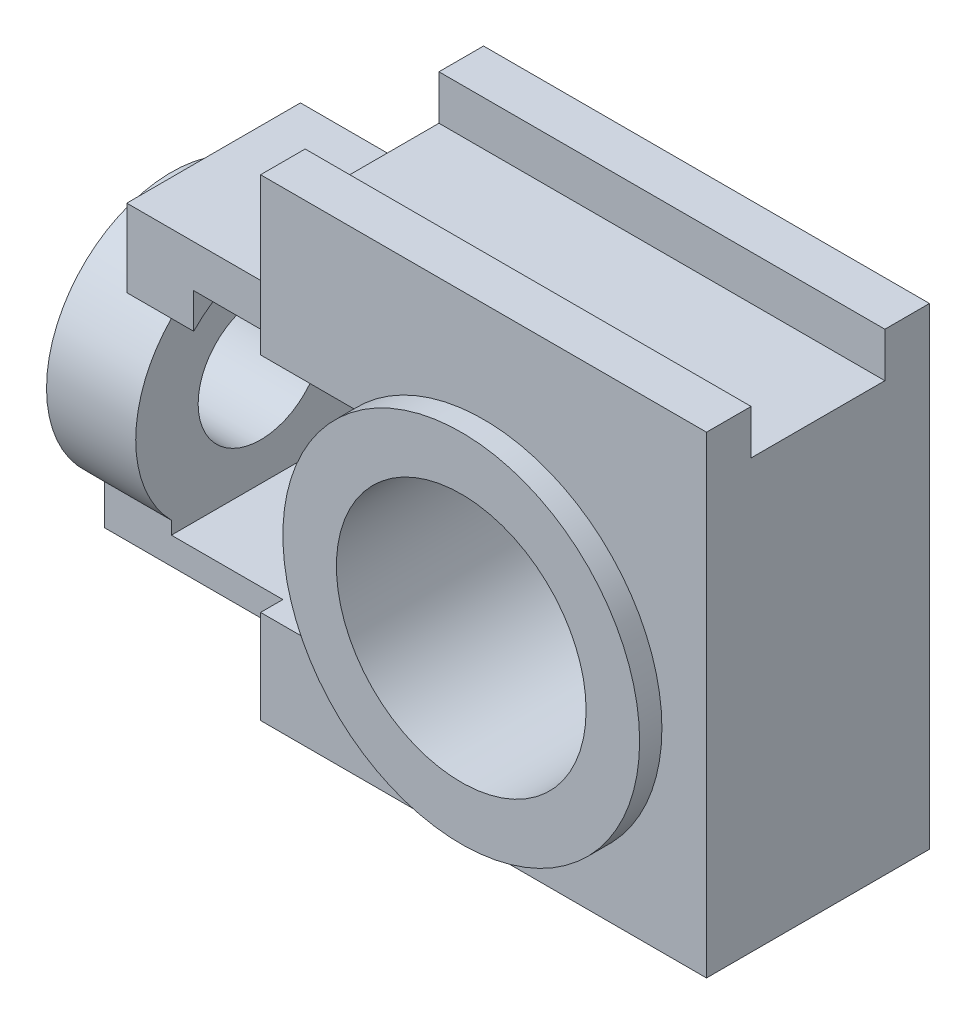
ISO-10303-21;
HEADER;
FILE_DESCRIPTION(('STEP AP214'),'2;1');
FILE_NAME('part.step','',(''),(''),'','','');
FILE_SCHEMA(('AUTOMOTIVE_DESIGN { 1 0 10303 214 1 1 1 1 }'));
ENDSEC;
DATA;
#1=APPLICATION_CONTEXT('core data for automotive mechanical design processes');
#2=APPLICATION_PROTOCOL_DEFINITION('international standard','automotive_design',2000,#1);
#3=PRODUCT_CONTEXT('',#1,'mechanical');
#4=PRODUCT('Part','Part','',(#3));
#5=PRODUCT_RELATED_PRODUCT_CATEGORY('part','',(#4));
#6=PRODUCT_DEFINITION_FORMATION('','',#4);
#7=PRODUCT_DEFINITION_CONTEXT('part definition',#1,'design');
#8=PRODUCT_DEFINITION('design','',#6,#7);
#9=PRODUCT_DEFINITION_SHAPE('','',#8);
#10=(LENGTH_UNIT() NAMED_UNIT(*) SI_UNIT(.MILLI.,.METRE.));
#11=(NAMED_UNIT(*) PLANE_ANGLE_UNIT() SI_UNIT($,.RADIAN.));
#12=(NAMED_UNIT(*) SI_UNIT($,.STERADIAN.) SOLID_ANGLE_UNIT());
#13=UNCERTAINTY_MEASURE_WITH_UNIT(LENGTH_MEASURE(1.E-05),#10,'distance_accuracy_value','');
#14=(GEOMETRIC_REPRESENTATION_CONTEXT(3) GLOBAL_UNCERTAINTY_ASSIGNED_CONTEXT((#13)) GLOBAL_UNIT_ASSIGNED_CONTEXT((#10,
#11,#12)) REPRESENTATION_CONTEXT('',''));
#15=CARTESIAN_POINT('',(0.,0.,0.));
#16=DIRECTION('',(0.,0.,1.));
#17=DIRECTION('',(1.,0.,0.));
#18=AXIS2_PLACEMENT_3D('',#15,#16,#17);
#19=CARTESIAN_POINT('',(0.,21.,0.));
#20=DIRECTION('',(0.,1.,0.));
#21=DIRECTION('',(0.,0.,1.));
#22=AXIS2_PLACEMENT_3D('',#19,#20,#21);
#23=PLANE('',#22);
#24=DIRECTION('',(1.,0.,0.));
#25=VECTOR('',#24,1.);
#26=CARTESIAN_POINT('',(-90.,21.,-20.));
#27=LINE('',#26,#25);
#28=CARTESIAN_POINT('',(-75.,21.,-20.));
#29=VERTEX_POINT('',#28);
#30=CARTESIAN_POINT('',(-50.,21.,-20.));
#31=VERTEX_POINT('',#30);
#32=EDGE_CURVE('E417',#29,#31,#27,.T.);
#33=ORIENTED_EDGE('',*,*,#32,.F.);
#34=DIRECTION('',(0.,0.,1.));
#35=VECTOR('',#34,1.);
#36=CARTESIAN_POINT('',(-75.,21.,0.));
#37=LINE('',#36,#35);
#38=CARTESIAN_POINT('',(-75.,21.,20.));
#39=VERTEX_POINT('',#38);
#40=EDGE_CURVE('E446',#29,#39,#37,.T.);
#41=ORIENTED_EDGE('',*,*,#40,.T.);
#42=DIRECTION('',(1.,0.,0.));
#43=VECTOR('',#42,1.);
#44=CARTESIAN_POINT('',(-90.,21.,20.));
#45=LINE('',#44,#43);
#46=CARTESIAN_POINT('',(-50.,21.,20.));
#47=VERTEX_POINT('',#46);
#48=EDGE_CURVE('E252',#39,#47,#45,.T.);
#49=ORIENTED_EDGE('',*,*,#48,.T.);
#50=DIRECTION('',(0.,0.,1.));
#51=VECTOR('',#50,1.);
#52=CARTESIAN_POINT('',(-50.,21.,-25.));
#53=LINE('',#52,#51);
#54=CARTESIAN_POINT('',(-50.,21.,25.));
#55=VERTEX_POINT('',#54);
#56=EDGE_CURVE('E423',#47,#55,#53,.T.);
#57=ORIENTED_EDGE('',*,*,#56,.T.);
#58=DIRECTION('',(1.,0.,0.));
#59=VECTOR('',#58,1.);
#60=CARTESIAN_POINT('',(-50.,21.,25.));
#61=LINE('',#60,#59);
#62=CARTESIAN_POINT('',(-33.0718913883074,21.,25.));
#63=VERTEX_POINT('',#62);
#64=EDGE_CURVE('E428',#55,#63,#61,.T.);
#65=ORIENTED_EDGE('',*,*,#64,.T.);
#66=DIRECTION('',(0.,0.,1.));
#67=VECTOR('',#66,1.);
#68=CARTESIAN_POINT('',(-33.0718913883074,21.,-25.));
#69=LINE('',#68,#67);
#70=CARTESIAN_POINT('',(-33.0718913883074,21.,-25.));
#71=VERTEX_POINT('',#70);
#72=EDGE_CURVE('E452',#71,#63,#69,.T.);
#73=ORIENTED_EDGE('',*,*,#72,.F.);
#74=DIRECTION('',(-1.,0.,0.));
#75=VECTOR('',#74,1.);
#76=CARTESIAN_POINT('',(50.,21.,-25.));
#77=LINE('',#76,#75);
#78=CARTESIAN_POINT('',(-50.,21.,-25.));
#79=VERTEX_POINT('',#78);
#80=EDGE_CURVE('E416',#71,#79,#77,.T.);
#81=ORIENTED_EDGE('',*,*,#80,.T.);
#82=EDGE_CURVE('E421',#79,#31,#53,.T.);
#83=ORIENTED_EDGE('',*,*,#82,.T.);
#84=EDGE_LOOP('',(#33,#41,#49,#57,#65,#73,#81,#83));
#85=FACE_BOUND('',#84,.T.);
#86=ADVANCED_FACE('F50',(#85),#23,.T.);
#87=CARTESIAN_POINT('',(-50.,106.,-25.));
#88=DIRECTION('',(-1.,0.,0.));
#89=DIRECTION('',(0.,-1.,0.));
#90=AXIS2_PLACEMENT_3D('',#87,#88,#89);
#91=PLANE('',#90);
#92=DIRECTION('',(0.,0.,1.));
#93=VECTOR('',#92,1.);
#94=CARTESIAN_POINT('',(-50.,71.,-25.));
#95=LINE('',#94,#93);
#96=CARTESIAN_POINT('',(-50.,71.,-19.0946483751058));
#97=VERTEX_POINT('',#96);
#98=CARTESIAN_POINT('',(-50.,71.,20.));
#99=VERTEX_POINT('',#98);
#100=EDGE_CURVE('E368',#97,#99,#95,.T.);
#101=ORIENTED_EDGE('',*,*,#100,.T.);
#102=DIRECTION('',(0.,-0.00096236717076537,0.999999536924607));
#103=VECTOR('',#102,1.);
#104=CARTESIAN_POINT('',(-50.,71.,20.));
#105=LINE('',#104,#103);
#106=CARTESIAN_POINT('',(-50.,71.0142498881101,5.19288485281843));
#107=VERTEX_POINT('',#106);
#108=EDGE_CURVE('E262',#107,#99,#105,.T.);
#109=ORIENTED_EDGE('',*,*,#108,.F.);
#110=CARTESIAN_POINT('',(-50.,43.5,0.));
#111=DIRECTION('',(1.,0.,0.));
#112=DIRECTION('',(0.,-1.,0.));
#113=AXIS2_PLACEMENT_3D('',#110,#111,#112);
#114=CIRCLE('',#113,28.);
#115=CARTESIAN_POINT('',(-50.,71.0142498881101,-5.19288485281842));
#116=VERTEX_POINT('',#115);
#117=EDGE_CURVE('E304',#116,#107,#114,.T.);
#118=ORIENTED_EDGE('',*,*,#117,.F.);
#119=DIRECTION('',(0.,0.00102504121876831,0.999999474645112));
#120=VECTOR('',#119,1.);
#121=CARTESIAN_POINT('',(-50.,71.,-19.0946483751058));
#122=LINE('',#121,#120);
#123=EDGE_CURVE('E266',#97,#116,#122,.T.);
#124=ORIENTED_EDGE('',*,*,#123,.F.);
#125=EDGE_LOOP('',(#101,#109,#118,#124));
#126=FACE_BOUND('',#125,.T.);
#127=ADVANCED_FACE('F506',(#126),#91,.T.);
#128=CARTESIAN_POINT('',(-50.,71.,-25.));
#129=VERTEX_POINT('',#128);
#130=EDGE_CURVE('E362',#129,#97,#95,.T.);
#131=ORIENTED_EDGE('',*,*,#130,.T.);
#132=DIRECTION('',(0.,-0.999869604471374,-0.0161485000621516));
#133=VECTOR('',#132,1.);
#134=CARTESIAN_POINT('',(-50.,80.4842706996611,-18.9414716555636));
#135=LINE('',#134,#133);
#136=CARTESIAN_POINT('',(-50.,80.4842706996611,-18.9414716555636));
#137=VERTEX_POINT('',#136);
#138=EDGE_CURVE('E305',#137,#97,#135,.T.);
#139=ORIENTED_EDGE('',*,*,#138,.F.);
#140=DIRECTION('',(0.,0.,-1.));
#141=VECTOR('',#140,1.);
#142=CARTESIAN_POINT('',(-50.,80.4842706996611,20.));
#143=LINE('',#142,#141);
#144=CARTESIAN_POINT('',(-50.,80.4842706996611,20.));
#145=VERTEX_POINT('',#144);
#146=EDGE_CURVE('E275',#145,#137,#143,.T.);
#147=ORIENTED_EDGE('',*,*,#146,.F.);
#148=DIRECTION('',(0.,1.,0.));
#149=VECTOR('',#148,1.);
#150=CARTESIAN_POINT('',(-50.,63.0959179422654,20.));
#151=LINE('',#150,#149);
#152=EDGE_CURVE('E293',#99,#145,#151,.T.);
#153=ORIENTED_EDGE('',*,*,#152,.F.);
#154=CARTESIAN_POINT('',(-50.,71.,25.));
#155=VERTEX_POINT('',#154);
#156=EDGE_CURVE('E367',#99,#155,#95,.T.);
#157=ORIENTED_EDGE('',*,*,#156,.T.);
#158=DIRECTION('',(0.,-1.,0.));
#159=VECTOR('',#158,1.);
#160=CARTESIAN_POINT('',(-50.,106.,25.));
#161=LINE('',#160,#159);
#162=CARTESIAN_POINT('',(-50.,106.,25.));
#163=VERTEX_POINT('',#162);
#164=EDGE_CURVE('E358',#163,#155,#161,.T.);
#165=ORIENTED_EDGE('',*,*,#164,.F.);
#166=DIRECTION('',(0.,0.,1.));
#167=VECTOR('',#166,1.);
#168=CARTESIAN_POINT('',(-50.,106.,-25.));
#169=LINE('',#168,#167);
#170=CARTESIAN_POINT('',(-50.,106.,15.));
#171=VERTEX_POINT('',#170);
#172=EDGE_CURVE('E373',#171,#163,#169,.T.);
#173=ORIENTED_EDGE('',*,*,#172,.F.);
#174=DIRECTION('',(0.,-1.,0.));
#175=VECTOR('',#174,1.);
#176=CARTESIAN_POINT('',(-50.,106.,15.));
#177=LINE('',#176,#175);
#178=CARTESIAN_POINT('',(-50.,96.,15.));
#179=VERTEX_POINT('',#178);
#180=EDGE_CURVE('E454',#171,#179,#177,.T.);
#181=ORIENTED_EDGE('',*,*,#180,.T.);
#182=DIRECTION('',(0.,0.,-1.));
#183=VECTOR('',#182,1.);
#184=CARTESIAN_POINT('',(-50.,96.,-25.));
#185=LINE('',#184,#183);
#186=CARTESIAN_POINT('',(-50.,96.,-15.));
#187=VERTEX_POINT('',#186);
#188=EDGE_CURVE('E54',#179,#187,#185,.T.);
#189=ORIENTED_EDGE('',*,*,#188,.T.);
#190=DIRECTION('',(0.,1.,0.));
#191=VECTOR('',#190,1.);
#192=CARTESIAN_POINT('',(-50.,106.,-15.));
#193=LINE('',#192,#191);
#194=CARTESIAN_POINT('',(-50.,106.,-15.));
#195=VERTEX_POINT('',#194);
#196=EDGE_CURVE('E11',#187,#195,#193,.T.);
#197=ORIENTED_EDGE('',*,*,#196,.T.);
#198=CARTESIAN_POINT('',(-50.,106.,-25.));
#199=VERTEX_POINT('',#198);
#200=EDGE_CURVE('E369',#199,#195,#169,.T.);
#201=ORIENTED_EDGE('',*,*,#200,.F.);
#202=DIRECTION('',(0.,-1.,0.));
#203=VECTOR('',#202,1.);
#204=CARTESIAN_POINT('',(-50.,106.,-25.));
#205=LINE('',#204,#203);
#206=EDGE_CURVE('E347',#199,#129,#205,.T.);
#207=ORIENTED_EDGE('',*,*,#206,.T.);
#208=EDGE_LOOP('',(#131,#139,#147,#153,#157,#165,#173,#181,#189,#197,#201,#207));
#209=FACE_BOUND('',#208,.T.);
#210=ADVANCED_FACE('F460',(#209),#91,.T.);
#211=CARTESIAN_POINT('',(-75.,43.5,0.));
#212=DIRECTION('',(-1.,0.,0.));
#213=DIRECTION('',(0.,0.,1.));
#214=AXIS2_PLACEMENT_3D('',#211,#212,#213);
#215=CYLINDRICAL_SURFACE('',#214,28.);
#216=DIRECTION('',(-1.,0.,0.));
#217=VECTOR('',#216,1.);
#218=CARTESIAN_POINT('',(-75.,23.9040820577346,20.));
#219=LINE('',#218,#217);
#220=CARTESIAN_POINT('',(-75.,23.9040820577346,20.));
#221=VERTEX_POINT('',#220);
#222=CARTESIAN_POINT('',(-90.,23.9040820577346,20.));
#223=VERTEX_POINT('',#222);
#224=EDGE_CURVE('E239',#221,#223,#219,.T.);
#225=ORIENTED_EDGE('',*,*,#224,.F.);
#226=CARTESIAN_POINT('',(-75.,43.5,0.));
#227=DIRECTION('',(-1.,0.,0.));
#228=DIRECTION('',(0.,0.,1.));
#229=AXIS2_PLACEMENT_3D('',#226,#227,#228);
#230=CIRCLE('',#229,28.);
#231=CARTESIAN_POINT('',(-75.,63.0959179422654,20.));
#232=VERTEX_POINT('',#231);
#233=EDGE_CURVE('E226',#221,#232,#230,.T.);
#234=ORIENTED_EDGE('',*,*,#233,.T.);
#235=DIRECTION('',(1.,0.,0.));
#236=VECTOR('',#235,1.);
#237=CARTESIAN_POINT('',(-85.,63.0959179422654,20.));
#238=LINE('',#237,#236);
#239=CARTESIAN_POINT('',(-85.,63.0959179422654,20.));
#240=VERTEX_POINT('',#239);
#241=EDGE_CURVE('E312',#240,#232,#238,.T.);
#242=ORIENTED_EDGE('',*,*,#241,.F.);
#243=CARTESIAN_POINT('',(-85.,43.5,0.));
#244=DIRECTION('',(1.,0.,0.));
#245=DIRECTION('',(0.,-1.,0.));
#246=AXIS2_PLACEMENT_3D('',#243,#244,#245);
#247=CIRCLE('',#246,28.);
#248=CARTESIAN_POINT('',(-85.,63.8711614859976,-19.2097834373896));
#249=VERTEX_POINT('',#248);
#250=EDGE_CURVE('E295',#249,#240,#247,.T.);
#251=ORIENTED_EDGE('',*,*,#250,.F.);
#252=DIRECTION('',(1.,0.,0.));
#253=VECTOR('',#252,1.);
#254=CARTESIAN_POINT('',(-85.,63.8711614859976,-19.2097834373896));
#255=LINE('',#254,#253);
#256=CARTESIAN_POINT('',(-75.,63.8711614859976,-19.2097834373896));
#257=VERTEX_POINT('',#256);
#258=EDGE_CURVE('E320',#249,#257,#255,.T.);
#259=ORIENTED_EDGE('',*,*,#258,.T.);
#260=CARTESIAN_POINT('',(-75.,23.9040820577346,-20.));
#261=VERTEX_POINT('',#260);
#262=EDGE_CURVE('E238',#257,#261,#230,.T.);
#263=ORIENTED_EDGE('',*,*,#262,.T.);
#264=DIRECTION('',(-1.,0.,0.));
#265=VECTOR('',#264,1.);
#266=CARTESIAN_POINT('',(-75.,23.9040820577346,-20.));
#267=LINE('',#266,#265);
#268=CARTESIAN_POINT('',(-90.,23.9040820577346,-20.));
#269=VERTEX_POINT('',#268);
#270=EDGE_CURVE('E244',#261,#269,#267,.T.);
#271=ORIENTED_EDGE('',*,*,#270,.T.);
#272=CARTESIAN_POINT('',(-90.,43.5,0.));
#273=DIRECTION('',(-1.,0.,0.));
#274=DIRECTION('',(0.,0.,1.));
#275=AXIS2_PLACEMENT_3D('',#272,#273,#274);
#276=CIRCLE('',#275,28.);
#277=EDGE_CURVE('E65',#269,#223,#276,.T.);
#278=ORIENTED_EDGE('',*,*,#277,.T.);
#279=EDGE_LOOP('',(#225,#234,#242,#251,#259,#263,#271,#278));
#280=FACE_BOUND('',#279,.T.);
#281=CARTESIAN_POINT('',(-95.,43.5,0.));
#282=DIRECTION('',(-1.,0.,0.));
#283=DIRECTION('',(0.,0.,1.));
#284=AXIS2_PLACEMENT_3D('',#281,#282,#283);
#285=CIRCLE('',#284,28.);
#286=CARTESIAN_POINT('',(-95.,43.5,28.));
#287=VERTEX_POINT('',#286);
#288=EDGE_CURVE('E395',#287,#287,#285,.T.);
#289=ORIENTED_EDGE('',*,*,#288,.F.);
#290=EDGE_LOOP('',(#289));
#291=FACE_BOUND('',#290,.T.);
#292=ADVANCED_FACE('F241',(#280,#291),#215,.T.);
#293=CARTESIAN_POINT('',(50.,106.,-25.));
#294=DIRECTION('',(0.,1.,0.));
#295=DIRECTION('',(-1.,0.,0.));
#296=AXIS2_PLACEMENT_3D('',#293,#294,#295);
#297=PLANE('',#296);
#298=DIRECTION('',(0.,0.,1.));
#299=VECTOR('',#298,1.);
#300=CARTESIAN_POINT('',(50.,106.,-25.));
#301=LINE('',#300,#299);
#302=CARTESIAN_POINT('',(50.,106.,15.));
#303=VERTEX_POINT('',#302);
#304=CARTESIAN_POINT('',(50.,106.,25.));
#305=VERTEX_POINT('',#304);
#306=EDGE_CURVE('E355',#303,#305,#301,.T.);
#307=ORIENTED_EDGE('',*,*,#306,.F.);
#308=DIRECTION('',(-1.,0.,0.));
#309=VECTOR('',#308,1.);
#310=CARTESIAN_POINT('',(389.772190337595,106.,15.));
#311=LINE('',#310,#309);
#312=EDGE_CURVE('E334',#303,#171,#311,.T.);
#313=ORIENTED_EDGE('',*,*,#312,.T.);
#314=ORIENTED_EDGE('',*,*,#172,.T.);
#315=DIRECTION('',(-1.,0.,0.));
#316=VECTOR('',#315,1.);
#317=CARTESIAN_POINT('',(50.,106.,25.));
#318=LINE('',#317,#316);
#319=EDGE_CURVE('E345',#305,#163,#318,.T.);
#320=ORIENTED_EDGE('',*,*,#319,.F.);
#321=EDGE_LOOP('',(#307,#313,#314,#320));
#322=FACE_BOUND('',#321,.T.);
#323=ADVANCED_FACE('F570',(#322),#297,.T.);
#324=CARTESIAN_POINT('',(-50.,21.,-25.));
#325=DIRECTION('',(1.,0.,0.));
#326=DIRECTION('',(0.,0.,-1.));
#327=AXIS2_PLACEMENT_3D('',#324,#325,#326);
#328=PLANE('',#327);
#329=DIRECTION('',(0.,1.,0.));
#330=VECTOR('',#329,1.);
#331=CARTESIAN_POINT('',(-50.,14.9431793908785,20.));
#332=LINE('',#331,#330);
#333=CARTESIAN_POINT('',(-50.,14.9431793908785,20.));
#334=VERTEX_POINT('',#333);
#335=EDGE_CURVE('E402',#334,#47,#332,.T.);
#336=ORIENTED_EDGE('',*,*,#335,.F.);
#337=DIRECTION('',(0.,0.,1.));
#338=VECTOR('',#337,1.);
#339=CARTESIAN_POINT('',(-50.,14.9431793908785,-20.));
#340=LINE('',#339,#338);
#341=CARTESIAN_POINT('',(-50.,14.9431793908785,-20.));
#342=VERTEX_POINT('',#341);
#343=EDGE_CURVE('E410',#342,#334,#340,.T.);
#344=ORIENTED_EDGE('',*,*,#343,.F.);
#345=DIRECTION('',(0.,-1.,0.));
#346=VECTOR('',#345,1.);
#347=CARTESIAN_POINT('',(-50.,21.,-20.));
#348=LINE('',#347,#346);
#349=EDGE_CURVE('E236',#31,#342,#348,.T.);
#350=ORIENTED_EDGE('',*,*,#349,.F.);
#351=ORIENTED_EDGE('',*,*,#82,.F.);
#352=DIRECTION('',(0.,-1.,0.));
#353=VECTOR('',#352,1.);
#354=CARTESIAN_POINT('',(-50.,21.,-25.));
#355=LINE('',#354,#353);
#356=CARTESIAN_POINT('',(-50.,0.,-25.));
#357=VERTEX_POINT('',#356);
#358=EDGE_CURVE('E444',#79,#357,#355,.T.);
#359=ORIENTED_EDGE('',*,*,#358,.T.);
#360=DIRECTION('',(0.,0.,1.));
#361=VECTOR('',#360,1.);
#362=CARTESIAN_POINT('',(-50.,0.,-25.));
#363=LINE('',#362,#361);
#364=CARTESIAN_POINT('',(-50.,0.,25.));
#365=VERTEX_POINT('',#364);
#366=EDGE_CURVE('E435',#357,#365,#363,.T.);
#367=ORIENTED_EDGE('',*,*,#366,.T.);
#368=DIRECTION('',(0.,-1.,0.));
#369=VECTOR('',#368,1.);
#370=CARTESIAN_POINT('',(-50.,21.,25.));
#371=LINE('',#370,#369);
#372=EDGE_CURVE('E445',#55,#365,#371,.T.);
#373=ORIENTED_EDGE('',*,*,#372,.F.);
#374=ORIENTED_EDGE('',*,*,#56,.F.);
#375=EDGE_LOOP('',(#336,#344,#350,#351,#359,#367,#373,#374));
#376=FACE_BOUND('',#375,.T.);
#377=ADVANCED_FACE('F530',(#376),#328,.F.);
#378=CARTESIAN_POINT('',(50.,21.,-25.));
#379=DIRECTION('',(0.,0.,1.));
#380=DIRECTION('',(1.,0.,0.));
#381=AXIS2_PLACEMENT_3D('',#378,#379,#380);
#382=PLANE('',#381);
#383=ORIENTED_EDGE('',*,*,#80,.F.);
#384=CARTESIAN_POINT('',(0.,43.5,-25.));
#385=DIRECTION('',(0.,0.,1.));
#386=DIRECTION('',(1.,0.,0.));
#387=AXIS2_PLACEMENT_3D('',#384,#385,#386);
#388=CIRCLE('',#387,40.);
#389=CARTESIAN_POINT('',(-29.0473750965557,71.,-25.));
#390=VERTEX_POINT('',#389);
#391=EDGE_CURVE('E383',#390,#71,#388,.T.);
#392=ORIENTED_EDGE('',*,*,#391,.F.);
#393=DIRECTION('',(1.,0.,0.));
#394=VECTOR('',#393,1.);
#395=CARTESIAN_POINT('',(-50.,71.,-25.));
#396=LINE('',#395,#394);
#397=EDGE_CURVE('E348',#129,#390,#396,.T.);
#398=ORIENTED_EDGE('',*,*,#397,.F.);
#399=ORIENTED_EDGE('',*,*,#206,.F.);
#400=DIRECTION('',(-1.,0.,0.));
#401=VECTOR('',#400,1.);
#402=CARTESIAN_POINT('',(50.,106.,-25.));
#403=LINE('',#402,#401);
#404=CARTESIAN_POINT('',(50.,106.,-25.));
#405=VERTEX_POINT('',#404);
#406=EDGE_CURVE('E344',#405,#199,#403,.T.);
#407=ORIENTED_EDGE('',*,*,#406,.F.);
#408=DIRECTION('',(0.,-1.,0.));
#409=VECTOR('',#408,1.);
#410=CARTESIAN_POINT('',(50.,21.,-25.));
#411=LINE('',#410,#409);
#412=CARTESIAN_POINT('',(50.,0.,-25.));
#413=VERTEX_POINT('',#412);
#414=EDGE_CURVE('E429',#405,#413,#411,.T.);
#415=ORIENTED_EDGE('',*,*,#414,.T.);
#416=DIRECTION('',(-1.,0.,0.));
#417=VECTOR('',#416,1.);
#418=CARTESIAN_POINT('',(50.,0.,-25.));
#419=LINE('',#418,#417);
#420=EDGE_CURVE('E420',#413,#357,#419,.T.);
#421=ORIENTED_EDGE('',*,*,#420,.T.);
#422=ORIENTED_EDGE('',*,*,#358,.F.);
#423=EDGE_LOOP('',(#383,#392,#398,#399,#407,#415,#421,#422));
#424=FACE_BOUND('',#423,.T.);
#425=CARTESIAN_POINT('',(0.,43.5,-25.));
#426=DIRECTION('',(0.,0.,1.));
#427=DIRECTION('',(1.,0.,0.));
#428=AXIS2_PLACEMENT_3D('',#425,#426,#427);
#429=CIRCLE('',#428,28.);
#430=CARTESIAN_POINT('',(28.,43.5,-25.));
#431=VERTEX_POINT('',#430);
#432=EDGE_CURVE('E385',#431,#431,#429,.T.);
#433=ORIENTED_EDGE('',*,*,#432,.T.);
#434=EDGE_LOOP('',(#433));
#435=FACE_BOUND('',#434,.T.);
#436=ADVANCED_FACE('F47',(#424,#435),#382,.F.);
#437=CARTESIAN_POINT('',(-50.,21.,25.));
#438=DIRECTION('',(0.,0.,-1.));
#439=DIRECTION('',(-1.,0.,0.));
#440=AXIS2_PLACEMENT_3D('',#437,#438,#439);
#441=PLANE('',#440);
#442=DIRECTION('',(0.,-1.,0.));
#443=VECTOR('',#442,1.);
#444=CARTESIAN_POINT('',(50.,21.,25.));
#445=LINE('',#444,#443);
#446=CARTESIAN_POINT('',(50.,0.,25.));
#447=VERTEX_POINT('',#446);
#448=EDGE_CURVE('E437',#305,#447,#445,.T.);
#449=ORIENTED_EDGE('',*,*,#448,.F.);
#450=ORIENTED_EDGE('',*,*,#319,.T.);
#451=ORIENTED_EDGE('',*,*,#164,.T.);
#452=DIRECTION('',(1.,0.,0.));
#453=VECTOR('',#452,1.);
#454=CARTESIAN_POINT('',(-50.,71.,25.));
#455=LINE('',#454,#453);
#456=CARTESIAN_POINT('',(-29.0473750965557,71.,25.));
#457=VERTEX_POINT('',#456);
#458=EDGE_CURVE('E349',#155,#457,#455,.T.);
#459=ORIENTED_EDGE('',*,*,#458,.T.);
#460=CARTESIAN_POINT('',(0.,43.5,25.));
#461=DIRECTION('',(0.,0.,-1.));
#462=DIRECTION('',(-1.,0.,0.));
#463=AXIS2_PLACEMENT_3D('',#460,#461,#462);
#464=CIRCLE('',#463,40.);
#465=EDGE_CURVE('E390',#457,#63,#464,.T.);
#466=ORIENTED_EDGE('',*,*,#465,.T.);
#467=ORIENTED_EDGE('',*,*,#64,.F.);
#468=ORIENTED_EDGE('',*,*,#372,.T.);
#469=DIRECTION('',(1.,0.,0.));
#470=VECTOR('',#469,1.);
#471=CARTESIAN_POINT('',(-50.,0.,25.));
#472=LINE('',#471,#470);
#473=EDGE_CURVE('E432',#365,#447,#472,.T.);
#474=ORIENTED_EDGE('',*,*,#473,.T.);
#475=EDGE_LOOP('',(#449,#450,#451,#459,#466,#467,#468,#474));
#476=FACE_BOUND('',#475,.T.);
#477=ADVANCED_FACE('F563',(#476),#441,.F.);
#478=CARTESIAN_POINT('',(50.,21.,25.));
#479=DIRECTION('',(-1.,0.,0.));
#480=DIRECTION('',(0.,0.,1.));
#481=AXIS2_PLACEMENT_3D('',#478,#479,#480);
#482=PLANE('',#481);
#483=CARTESIAN_POINT('',(50.,106.,-15.));
#484=VERTEX_POINT('',#483);
#485=EDGE_CURVE('E372',#405,#484,#301,.T.);
#486=ORIENTED_EDGE('',*,*,#485,.T.);
#487=DIRECTION('',(0.,-1.,0.));
#488=VECTOR('',#487,1.);
#489=CARTESIAN_POINT('',(50.,96.,-15.));
#490=LINE('',#489,#488);
#491=CARTESIAN_POINT('',(50.,96.,-15.));
#492=VERTEX_POINT('',#491);
#493=EDGE_CURVE('E324',#484,#492,#490,.T.);
#494=ORIENTED_EDGE('',*,*,#493,.T.);
#495=DIRECTION('',(0.,0.,1.));
#496=VECTOR('',#495,1.);
#497=CARTESIAN_POINT('',(50.,96.,15.));
#498=LINE('',#497,#496);
#499=CARTESIAN_POINT('',(50.,96.,15.));
#500=VERTEX_POINT('',#499);
#501=EDGE_CURVE('E327',#492,#500,#498,.T.);
#502=ORIENTED_EDGE('',*,*,#501,.T.);
#503=DIRECTION('',(0.,1.,0.));
#504=VECTOR('',#503,1.);
#505=CARTESIAN_POINT('',(50.,106.,15.));
#506=LINE('',#505,#504);
#507=EDGE_CURVE('E326',#500,#303,#506,.T.);
#508=ORIENTED_EDGE('',*,*,#507,.T.);
#509=ORIENTED_EDGE('',*,*,#306,.T.);
#510=ORIENTED_EDGE('',*,*,#448,.T.);
#511=DIRECTION('',(0.,0.,-1.));
#512=VECTOR('',#511,1.);
#513=CARTESIAN_POINT('',(50.,0.,25.));
#514=LINE('',#513,#512);
#515=EDGE_CURVE('E422',#447,#413,#514,.T.);
#516=ORIENTED_EDGE('',*,*,#515,.T.);
#517=ORIENTED_EDGE('',*,*,#414,.F.);
#518=EDGE_LOOP('',(#486,#494,#502,#508,#509,#510,#516,#517));
#519=FACE_BOUND('',#518,.T.);
#520=ADVANCED_FACE('F466',(#519),#482,.F.);
#521=CARTESIAN_POINT('',(0.,0.,0.));
#522=DIRECTION('',(0.,1.,0.));
#523=DIRECTION('',(0.,0.,1.));
#524=AXIS2_PLACEMENT_3D('',#521,#522,#523);
#525=PLANE('',#524);
#526=ORIENTED_EDGE('',*,*,#420,.F.);
#527=ORIENTED_EDGE('',*,*,#515,.F.);
#528=ORIENTED_EDGE('',*,*,#473,.F.);
#529=ORIENTED_EDGE('',*,*,#366,.F.);
#530=EDGE_LOOP('',(#526,#527,#528,#529));
#531=FACE_BOUND('',#530,.T.);
#532=ADVANCED_FACE('F560',(#531),#525,.F.);
#533=CARTESIAN_POINT('',(-90.,21.,-20.));
#534=DIRECTION('',(0.,0.,1.));
#535=DIRECTION('',(1.,0.,0.));
#536=AXIS2_PLACEMENT_3D('',#533,#534,#535);
#537=PLANE('',#536);
#538=DIRECTION('',(0.,-1.,0.));
#539=VECTOR('',#538,1.);
#540=CARTESIAN_POINT('',(-90.,21.,-20.));
#541=LINE('',#540,#539);
#542=CARTESIAN_POINT('',(-90.,14.9431793908785,-20.));
#543=VERTEX_POINT('',#542);
#544=EDGE_CURVE('E68',#269,#543,#541,.T.);
#545=ORIENTED_EDGE('',*,*,#544,.F.);
#546=ORIENTED_EDGE('',*,*,#270,.F.);
#547=DIRECTION('',(0.,-1.,0.));
#548=VECTOR('',#547,1.);
#549=CARTESIAN_POINT('',(-75.,14.9431793908785,-20.));
#550=LINE('',#549,#548);
#551=EDGE_CURVE('E246',#261,#29,#550,.T.);
#552=ORIENTED_EDGE('',*,*,#551,.T.);
#553=ORIENTED_EDGE('',*,*,#32,.T.);
#554=ORIENTED_EDGE('',*,*,#349,.T.);
#555=DIRECTION('',(1.,0.,0.));
#556=VECTOR('',#555,1.);
#557=CARTESIAN_POINT('',(-90.,14.9431793908785,-20.));
#558=LINE('',#557,#556);
#559=EDGE_CURVE('E411',#543,#342,#558,.T.);
#560=ORIENTED_EDGE('',*,*,#559,.F.);
#561=EDGE_LOOP('',(#545,#546,#552,#553,#554,#560));
#562=FACE_BOUND('',#561,.T.);
#563=ADVANCED_FACE('F518',(#562),#537,.F.);
#564=CARTESIAN_POINT('',(-90.,14.9431793908785,-20.));
#565=DIRECTION('',(0.,1.,0.));
#566=DIRECTION('',(0.,0.,1.));
#567=AXIS2_PLACEMENT_3D('',#564,#565,#566);
#568=PLANE('',#567);
#569=ORIENTED_EDGE('',*,*,#559,.T.);
#570=ORIENTED_EDGE('',*,*,#343,.T.);
#571=DIRECTION('',(1.,0.,0.));
#572=VECTOR('',#571,1.);
#573=CARTESIAN_POINT('',(-90.,14.9431793908785,20.));
#574=LINE('',#573,#572);
#575=CARTESIAN_POINT('',(-90.,14.9431793908785,20.));
#576=VERTEX_POINT('',#575);
#577=EDGE_CURVE('E414',#576,#334,#574,.T.);
#578=ORIENTED_EDGE('',*,*,#577,.F.);
#579=DIRECTION('',(0.,0.,1.));
#580=VECTOR('',#579,1.);
#581=CARTESIAN_POINT('',(-90.,14.9431793908785,-20.));
#582=LINE('',#581,#580);
#583=EDGE_CURVE('E398',#543,#576,#582,.T.);
#584=ORIENTED_EDGE('',*,*,#583,.F.);
#585=EDGE_LOOP('',(#569,#570,#578,#584));
#586=FACE_BOUND('',#585,.T.);
#587=ADVANCED_FACE('F531',(#586),#568,.F.);
#588=CARTESIAN_POINT('',(-90.,14.9431793908785,20.));
#589=DIRECTION('',(0.,0.,-1.));
#590=DIRECTION('',(-1.,0.,0.));
#591=AXIS2_PLACEMENT_3D('',#588,#589,#590);
#592=PLANE('',#591);
#593=ORIENTED_EDGE('',*,*,#577,.T.);
#594=ORIENTED_EDGE('',*,*,#335,.T.);
#595=ORIENTED_EDGE('',*,*,#48,.F.);
#596=DIRECTION('',(0.,1.,0.));
#597=VECTOR('',#596,1.);
#598=CARTESIAN_POINT('',(-75.,14.9431793908785,20.));
#599=LINE('',#598,#597);
#600=EDGE_CURVE('E235',#39,#221,#599,.T.);
#601=ORIENTED_EDGE('',*,*,#600,.T.);
#602=ORIENTED_EDGE('',*,*,#224,.T.);
#603=DIRECTION('',(0.,1.,0.));
#604=VECTOR('',#603,1.);
#605=CARTESIAN_POINT('',(-90.,14.9431793908785,20.));
#606=LINE('',#605,#604);
#607=EDGE_CURVE('E401',#576,#223,#606,.T.);
#608=ORIENTED_EDGE('',*,*,#607,.F.);
#609=EDGE_LOOP('',(#593,#594,#595,#601,#602,#608));
#610=FACE_BOUND('',#609,.T.);
#611=ADVANCED_FACE('F248',(#610),#592,.F.);
#612=CARTESIAN_POINT('',(-90.,0.,0.));
#613=DIRECTION('',(-1.,0.,0.));
#614=DIRECTION('',(0.,0.,1.));
#615=AXIS2_PLACEMENT_3D('',#612,#613,#614);
#616=PLANE('',#615);
#617=ORIENTED_EDGE('',*,*,#277,.F.);
#618=ORIENTED_EDGE('',*,*,#544,.T.);
#619=ORIENTED_EDGE('',*,*,#583,.T.);
#620=ORIENTED_EDGE('',*,*,#607,.T.);
#621=EDGE_LOOP('',(#617,#618,#619,#620));
#622=FACE_BOUND('',#621,.T.);
#623=ADVANCED_FACE('F537',(#622),#616,.T.);
#624=CARTESIAN_POINT('',(-75.,43.5,0.));
#625=DIRECTION('',(-1.,0.,0.));
#626=DIRECTION('',(0.,0.,1.));
#627=AXIS2_PLACEMENT_3D('',#624,#625,#626);
#628=PLANE('',#627);
#629=ORIENTED_EDGE('',*,*,#40,.F.);
#630=ORIENTED_EDGE('',*,*,#551,.F.);
#631=ORIENTED_EDGE('',*,*,#262,.F.);
#632=EDGE_CURVE('E234',#232,#257,#230,.T.);
#633=ORIENTED_EDGE('',*,*,#632,.F.);
#634=ORIENTED_EDGE('',*,*,#233,.F.);
#635=ORIENTED_EDGE('',*,*,#600,.F.);
#636=EDGE_LOOP('',(#629,#630,#631,#633,#634,#635));
#637=FACE_BOUND('',#636,.T.);
#638=CARTESIAN_POINT('',(-75.,43.5,0.));
#639=DIRECTION('',(-1.,0.,0.));
#640=DIRECTION('',(0.,0.,1.));
#641=AXIS2_PLACEMENT_3D('',#638,#639,#640);
#642=CIRCLE('',#641,14.);
#643=CARTESIAN_POINT('',(-75.,43.5,14.));
#644=VERTEX_POINT('',#643);
#645=EDGE_CURVE('E397',#644,#644,#642,.T.);
#646=ORIENTED_EDGE('',*,*,#645,.T.);
#647=EDGE_LOOP('',(#646));
#648=FACE_BOUND('',#647,.T.);
#649=ADVANCED_FACE('F230',(#637,#648),#628,.F.);
#650=CARTESIAN_POINT('',(-75.,43.5,0.));
#651=DIRECTION('',(-1.,0.,0.));
#652=DIRECTION('',(0.,0.,1.));
#653=AXIS2_PLACEMENT_3D('',#650,#651,#652);
#654=CYLINDRICAL_SURFACE('',#653,14.);
#655=ORIENTED_EDGE('',*,*,#645,.F.);
#656=EDGE_LOOP('',(#655));
#657=FACE_BOUND('',#656,.T.);
#658=CARTESIAN_POINT('',(-95.,43.5,0.));
#659=DIRECTION('',(-1.,0.,0.));
#660=DIRECTION('',(0.,0.,1.));
#661=AXIS2_PLACEMENT_3D('',#658,#659,#660);
#662=CIRCLE('',#661,14.);
#663=CARTESIAN_POINT('',(-95.,43.5,14.));
#664=VERTEX_POINT('',#663);
#665=EDGE_CURVE('E388',#664,#664,#662,.T.);
#666=ORIENTED_EDGE('',*,*,#665,.T.);
#667=EDGE_LOOP('',(#666));
#668=FACE_BOUND('',#667,.T.);
#669=ADVANCED_FACE('F545',(#657,#668),#654,.F.);
#670=CARTESIAN_POINT('',(-95.,43.5,0.));
#671=DIRECTION('',(-1.,0.,0.));
#672=DIRECTION('',(0.,0.,1.));
#673=AXIS2_PLACEMENT_3D('',#670,#671,#672);
#674=PLANE('',#673);
#675=ORIENTED_EDGE('',*,*,#288,.T.);
#676=EDGE_LOOP('',(#675));
#677=FACE_BOUND('',#676,.T.);
#678=ORIENTED_EDGE('',*,*,#665,.F.);
#679=EDGE_LOOP('',(#678));
#680=FACE_BOUND('',#679,.T.);
#681=ADVANCED_FACE('F777',(#677,#680),#674,.T.);
#682=CARTESIAN_POINT('',(0.,43.5,-25.));
#683=DIRECTION('',(0.,0.,1.));
#684=DIRECTION('',(1.,0.,0.));
#685=AXIS2_PLACEMENT_3D('',#682,#683,#684);
#686=CYLINDRICAL_SURFACE('',#685,40.);
#687=DIRECTION('',(0.,0.,1.));
#688=VECTOR('',#687,1.);
#689=CARTESIAN_POINT('',(-29.0473750965557,71.,-25.));
#690=LINE('',#689,#688);
#691=EDGE_CURVE('E363',#390,#457,#690,.T.);
#692=ORIENTED_EDGE('',*,*,#691,.F.);
#693=ORIENTED_EDGE('',*,*,#391,.T.);
#694=ORIENTED_EDGE('',*,*,#72,.T.);
#695=ORIENTED_EDGE('',*,*,#465,.F.);
#696=EDGE_LOOP('',(#692,#693,#694,#695));
#697=FACE_BOUND('',#696,.T.);
#698=CARTESIAN_POINT('',(0.,43.5,30.));
#699=DIRECTION('',(0.,0.,1.));
#700=DIRECTION('',(1.,0.,0.));
#701=AXIS2_PLACEMENT_3D('',#698,#699,#700);
#702=CIRCLE('',#701,40.);
#703=CARTESIAN_POINT('',(40.,43.5,30.));
#704=VERTEX_POINT('',#703);
#705=EDGE_CURVE('E378',#704,#704,#702,.T.);
#706=ORIENTED_EDGE('',*,*,#705,.F.);
#707=EDGE_LOOP('',(#706));
#708=FACE_BOUND('',#707,.T.);
#709=ADVANCED_FACE('F769',(#697,#708),#686,.T.);
#710=CARTESIAN_POINT('',(0.,43.5,-25.));
#711=DIRECTION('',(0.,0.,1.));
#712=DIRECTION('',(1.,0.,0.));
#713=AXIS2_PLACEMENT_3D('',#710,#711,#712);
#714=CYLINDRICAL_SURFACE('',#713,28.);
#715=ORIENTED_EDGE('',*,*,#432,.F.);
#716=EDGE_LOOP('',(#715));
#717=FACE_BOUND('',#716,.T.);
#718=CARTESIAN_POINT('',(0.,43.5,30.));
#719=DIRECTION('',(0.,0.,1.));
#720=DIRECTION('',(1.,0.,0.));
#721=AXIS2_PLACEMENT_3D('',#718,#719,#720);
#722=CIRCLE('',#721,28.);
#723=CARTESIAN_POINT('',(28.,43.5,30.));
#724=VERTEX_POINT('',#723);
#725=EDGE_CURVE('E364',#724,#724,#722,.T.);
#726=ORIENTED_EDGE('',*,*,#725,.T.);
#727=EDGE_LOOP('',(#726));
#728=FACE_BOUND('',#727,.T.);
#729=ADVANCED_FACE('F594',(#717,#728),#714,.F.);
#730=CARTESIAN_POINT('',(0.,43.5,30.));
#731=DIRECTION('',(0.,0.,1.));
#732=DIRECTION('',(1.,0.,0.));
#733=AXIS2_PLACEMENT_3D('',#730,#731,#732);
#734=PLANE('',#733);
#735=ORIENTED_EDGE('',*,*,#705,.T.);
#736=EDGE_LOOP('',(#735));
#737=FACE_BOUND('',#736,.T.);
#738=ORIENTED_EDGE('',*,*,#725,.F.);
#739=EDGE_LOOP('',(#738));
#740=FACE_BOUND('',#739,.T.);
#741=ADVANCED_FACE('F589',(#737,#740),#734,.T.);
#742=CARTESIAN_POINT('',(-50.,71.,-25.));
#743=DIRECTION('',(0.,-1.,0.));
#744=DIRECTION('',(0.,0.,-1.));
#745=AXIS2_PLACEMENT_3D('',#742,#743,#744);
#746=PLANE('',#745);
#747=ORIENTED_EDGE('',*,*,#458,.F.);
#748=ORIENTED_EDGE('',*,*,#156,.F.);
#749=ORIENTED_EDGE('',*,*,#100,.F.);
#750=ORIENTED_EDGE('',*,*,#130,.F.);
#751=ORIENTED_EDGE('',*,*,#397,.T.);
#752=ORIENTED_EDGE('',*,*,#691,.T.);
#753=EDGE_LOOP('',(#747,#748,#749,#750,#751,#752));
#754=FACE_BOUND('',#753,.T.);
#755=ADVANCED_FACE('F578',(#754),#746,.T.);
#756=DIRECTION('',(-1.,0.,0.));
#757=VECTOR('',#756,1.);
#758=CARTESIAN_POINT('',(389.772190337595,106.,-15.));
#759=LINE('',#758,#757);
#760=EDGE_CURVE('E340',#484,#195,#759,.T.);
#761=ORIENTED_EDGE('',*,*,#760,.F.);
#762=ORIENTED_EDGE('',*,*,#485,.F.);
#763=ORIENTED_EDGE('',*,*,#406,.T.);
#764=ORIENTED_EDGE('',*,*,#200,.T.);
#765=EDGE_LOOP('',(#761,#762,#763,#764));
#766=FACE_BOUND('',#765,.T.);
#767=ADVANCED_FACE('F475',(#766),#297,.T.);
#768=CARTESIAN_POINT('',(389.772190337595,96.,-15.));
#769=DIRECTION('',(0.,0.,1.));
#770=DIRECTION('',(0.,-1.,0.));
#771=AXIS2_PLACEMENT_3D('',#768,#769,#770);
#772=PLANE('',#771);
#773=ORIENTED_EDGE('',*,*,#196,.F.);
#774=DIRECTION('',(-1.,0.,0.));
#775=VECTOR('',#774,1.);
#776=CARTESIAN_POINT('',(389.772190337595,96.,-15.));
#777=LINE('',#776,#775);
#778=EDGE_CURVE('E339',#492,#187,#777,.T.);
#779=ORIENTED_EDGE('',*,*,#778,.F.);
#780=ORIENTED_EDGE('',*,*,#493,.F.);
#781=ORIENTED_EDGE('',*,*,#760,.T.);
#782=EDGE_LOOP('',(#773,#779,#780,#781));
#783=FACE_BOUND('',#782,.T.);
#784=ADVANCED_FACE('F463',(#783),#772,.T.);
#785=CARTESIAN_POINT('',(389.772190337595,96.,15.));
#786=DIRECTION('',(0.,1.,0.));
#787=DIRECTION('',(0.,0.,1.));
#788=AXIS2_PLACEMENT_3D('',#785,#786,#787);
#789=PLANE('',#788);
#790=ORIENTED_EDGE('',*,*,#188,.F.);
#791=DIRECTION('',(-1.,0.,0.));
#792=VECTOR('',#791,1.);
#793=CARTESIAN_POINT('',(389.772190337595,96.,15.));
#794=LINE('',#793,#792);
#795=EDGE_CURVE('E333',#500,#179,#794,.T.);
#796=ORIENTED_EDGE('',*,*,#795,.F.);
#797=ORIENTED_EDGE('',*,*,#501,.F.);
#798=ORIENTED_EDGE('',*,*,#778,.T.);
#799=EDGE_LOOP('',(#790,#796,#797,#798));
#800=FACE_BOUND('',#799,.T.);
#801=ADVANCED_FACE('F464',(#800),#789,.T.);
#802=CARTESIAN_POINT('',(389.772190337595,106.,15.));
#803=DIRECTION('',(0.,0.,-1.));
#804=DIRECTION('',(0.,1.,0.));
#805=AXIS2_PLACEMENT_3D('',#802,#803,#804);
#806=PLANE('',#805);
#807=ORIENTED_EDGE('',*,*,#180,.F.);
#808=ORIENTED_EDGE('',*,*,#312,.F.);
#809=ORIENTED_EDGE('',*,*,#507,.F.);
#810=ORIENTED_EDGE('',*,*,#795,.T.);
#811=EDGE_LOOP('',(#807,#808,#809,#810));
#812=FACE_BOUND('',#811,.T.);
#813=ADVANCED_FACE('F596',(#812),#806,.T.);
#814=CARTESIAN_POINT('',(-85.,43.5,0.));
#815=DIRECTION('',(1.,0.,0.));
#816=DIRECTION('',(0.,1.,0.));
#817=AXIS2_PLACEMENT_3D('',#814,#815,#816);
#818=CYLINDRICAL_SURFACE('',#817,28.);
#819=ORIENTED_EDGE('',*,*,#117,.T.);
#820=DIRECTION('',(1.,0.,0.));
#821=VECTOR('',#820,1.);
#822=CARTESIAN_POINT('',(-70.,71.0142498881101,5.19288485281843));
#823=LINE('',#822,#821);
#824=CARTESIAN_POINT('',(-70.,71.0142498881101,5.19288485281843));
#825=VERTEX_POINT('',#824);
#826=EDGE_CURVE('E268',#825,#107,#823,.T.);
#827=ORIENTED_EDGE('',*,*,#826,.F.);
#828=CARTESIAN_POINT('',(-70.,43.5,0.));
#829=DIRECTION('',(-1.,0.,0.));
#830=DIRECTION('',(0.,1.,0.));
#831=AXIS2_PLACEMENT_3D('',#828,#829,#830);
#832=CIRCLE('',#831,28.);
#833=CARTESIAN_POINT('',(-70.,63.0959179422654,20.));
#834=VERTEX_POINT('',#833);
#835=EDGE_CURVE('E265',#834,#825,#832,.T.);
#836=ORIENTED_EDGE('',*,*,#835,.F.);
#837=EDGE_CURVE('E315',#232,#834,#238,.T.);
#838=ORIENTED_EDGE('',*,*,#837,.F.);
#839=ORIENTED_EDGE('',*,*,#632,.T.);
#840=CARTESIAN_POINT('',(-70.,63.8711614859976,-19.2097834373896));
#841=VERTEX_POINT('',#840);
#842=EDGE_CURVE('E317',#257,#841,#255,.T.);
#843=ORIENTED_EDGE('',*,*,#842,.T.);
#844=CARTESIAN_POINT('',(-70.,43.5,0.));
#845=DIRECTION('',(-1.,0.,0.));
#846=DIRECTION('',(0.,1.,0.));
#847=AXIS2_PLACEMENT_3D('',#844,#845,#846);
#848=CIRCLE('',#847,28.);
#849=CARTESIAN_POINT('',(-70.,71.0142498881101,-5.19288485281842));
#850=VERTEX_POINT('',#849);
#851=EDGE_CURVE('E282',#850,#841,#848,.T.);
#852=ORIENTED_EDGE('',*,*,#851,.F.);
#853=DIRECTION('',(1.,0.,0.));
#854=VECTOR('',#853,1.);
#855=CARTESIAN_POINT('',(-70.,71.0142498881101,-5.19288485281842));
#856=LINE('',#855,#854);
#857=EDGE_CURVE('E257',#850,#116,#856,.T.);
#858=ORIENTED_EDGE('',*,*,#857,.T.);
#859=EDGE_LOOP('',(#819,#827,#836,#838,#839,#843,#852,#858));
#860=FACE_BOUND('',#859,.T.);
#861=ADVANCED_FACE('F508',(#860),#818,.F.);
#862=CARTESIAN_POINT('',(-85.,80.4842706996611,20.));
#863=DIRECTION('',(0.,-1.,0.));
#864=DIRECTION('',(1.,0.,0.));
#865=AXIS2_PLACEMENT_3D('',#862,#863,#864);
#866=PLANE('',#865);
#867=ORIENTED_EDGE('',*,*,#146,.T.);
#868=DIRECTION('',(1.,0.,0.));
#869=VECTOR('',#868,1.);
#870=CARTESIAN_POINT('',(-85.,80.4842706996611,-18.9414716555636));
#871=LINE('',#870,#869);
#872=CARTESIAN_POINT('',(-85.,80.4842706996611,-18.9414716555636));
#873=VERTEX_POINT('',#872);
#874=EDGE_CURVE('E318',#873,#137,#871,.T.);
#875=ORIENTED_EDGE('',*,*,#874,.F.);
#876=DIRECTION('',(0.,0.,-1.));
#877=VECTOR('',#876,1.);
#878=CARTESIAN_POINT('',(-85.,80.4842706996611,20.));
#879=LINE('',#878,#877);
#880=CARTESIAN_POINT('',(-85.,80.4842706996611,20.));
#881=VERTEX_POINT('',#880);
#882=EDGE_CURVE('E289',#881,#873,#879,.T.);
#883=ORIENTED_EDGE('',*,*,#882,.F.);
#884=DIRECTION('',(1.,0.,0.));
#885=VECTOR('',#884,1.);
#886=CARTESIAN_POINT('',(-85.,80.4842706996611,20.));
#887=LINE('',#886,#885);
#888=EDGE_CURVE('E299',#881,#145,#887,.T.);
#889=ORIENTED_EDGE('',*,*,#888,.T.);
#890=EDGE_LOOP('',(#867,#875,#883,#889));
#891=FACE_BOUND('',#890,.T.);
#892=ADVANCED_FACE('F489',(#891),#866,.F.);
#893=CARTESIAN_POINT('',(-85.,80.4842706996611,-18.9414716555636));
#894=DIRECTION('',(0.,-0.0161485000621516,0.999869604471375));
#895=DIRECTION('',(0.,-0.999869604471375,-0.0161485000621516));
#896=AXIS2_PLACEMENT_3D('',#893,#894,#895);
#897=PLANE('',#896);
#898=ORIENTED_EDGE('',*,*,#138,.T.);
#899=DIRECTION('',(1.,0.,0.));
#900=VECTOR('',#899,1.);
#901=CARTESIAN_POINT('',(-70.,71.,-19.0946483751058));
#902=LINE('',#901,#900);
#903=CARTESIAN_POINT('',(-70.,71.,-19.0946483751058));
#904=VERTEX_POINT('',#903);
#905=EDGE_CURVE('E273',#904,#97,#902,.T.);
#906=ORIENTED_EDGE('',*,*,#905,.F.);
#907=DIRECTION('',(0.,0.999869604471374,0.0161485000621517));
#908=VECTOR('',#907,1.);
#909=CARTESIAN_POINT('',(-70.,63.8711614859976,-19.2097834373896));
#910=LINE('',#909,#908);
#911=EDGE_CURVE('E281',#841,#904,#910,.T.);
#912=ORIENTED_EDGE('',*,*,#911,.F.);
#913=ORIENTED_EDGE('',*,*,#842,.F.);
#914=ORIENTED_EDGE('',*,*,#258,.F.);
#915=DIRECTION('',(0.,-0.999869604471374,-0.0161485000621516));
#916=VECTOR('',#915,1.);
#917=CARTESIAN_POINT('',(-85.,80.4842706996611,-18.9414716555636));
#918=LINE('',#917,#916);
#919=EDGE_CURVE('E288',#873,#249,#918,.T.);
#920=ORIENTED_EDGE('',*,*,#919,.F.);
#921=ORIENTED_EDGE('',*,*,#874,.T.);
#922=EDGE_LOOP('',(#898,#906,#912,#913,#914,#920,#921));
#923=FACE_BOUND('',#922,.T.);
#924=ADVANCED_FACE('F481',(#923),#897,.F.);
#925=CARTESIAN_POINT('',(-85.,63.0959179422654,20.));
#926=DIRECTION('',(0.,0.,-1.));
#927=DIRECTION('',(-1.,0.,0.));
#928=AXIS2_PLACEMENT_3D('',#925,#926,#927);
#929=PLANE('',#928);
#930=DIRECTION('',(0.,-1.,0.));
#931=VECTOR('',#930,1.);
#932=CARTESIAN_POINT('',(-70.,71.,20.));
#933=LINE('',#932,#931);
#934=CARTESIAN_POINT('',(-70.,71.,20.));
#935=VERTEX_POINT('',#934);
#936=EDGE_CURVE('E258',#935,#834,#933,.T.);
#937=ORIENTED_EDGE('',*,*,#936,.F.);
#938=DIRECTION('',(1.,0.,0.));
#939=VECTOR('',#938,1.);
#940=CARTESIAN_POINT('',(-70.,71.,20.));
#941=LINE('',#940,#939);
#942=EDGE_CURVE('E267',#935,#99,#941,.T.);
#943=ORIENTED_EDGE('',*,*,#942,.T.);
#944=ORIENTED_EDGE('',*,*,#152,.T.);
#945=ORIENTED_EDGE('',*,*,#888,.F.);
#946=DIRECTION('',(0.,1.,0.));
#947=VECTOR('',#946,1.);
#948=CARTESIAN_POINT('',(-85.,63.0959179422654,20.));
#949=LINE('',#948,#947);
#950=EDGE_CURVE('E300',#240,#881,#949,.T.);
#951=ORIENTED_EDGE('',*,*,#950,.F.);
#952=ORIENTED_EDGE('',*,*,#241,.T.);
#953=ORIENTED_EDGE('',*,*,#837,.T.);
#954=EDGE_LOOP('',(#937,#943,#944,#945,#951,#952,#953));
#955=FACE_BOUND('',#954,.T.);
#956=ADVANCED_FACE('F496',(#955),#929,.F.);
#957=CARTESIAN_POINT('',(-85.,43.5,0.));
#958=DIRECTION('',(-1.,0.,0.));
#959=DIRECTION('',(0.,-1.,0.));
#960=AXIS2_PLACEMENT_3D('',#957,#958,#959);
#961=PLANE('',#960);
#962=ORIENTED_EDGE('',*,*,#882,.T.);
#963=ORIENTED_EDGE('',*,*,#919,.T.);
#964=ORIENTED_EDGE('',*,*,#250,.T.);
#965=ORIENTED_EDGE('',*,*,#950,.T.);
#966=EDGE_LOOP('',(#962,#963,#964,#965));
#967=FACE_BOUND('',#966,.T.);
#968=ADVANCED_FACE('F606',(#967),#961,.T.);
#969=CARTESIAN_POINT('',(-70.,71.,20.));
#970=DIRECTION('',(0.,0.999999536924607,0.00096236717076537));
#971=DIRECTION('',(0.,-0.00096236717076537,0.999999536924607));
#972=AXIS2_PLACEMENT_3D('',#969,#970,#971);
#973=PLANE('',#972);
#974=ORIENTED_EDGE('',*,*,#108,.T.);
#975=ORIENTED_EDGE('',*,*,#942,.F.);
#976=DIRECTION('',(0.,-0.00096236717076537,0.999999536924607));
#977=VECTOR('',#976,1.);
#978=CARTESIAN_POINT('',(-70.,71.,20.));
#979=LINE('',#978,#977);
#980=EDGE_CURVE('E259',#825,#935,#979,.T.);
#981=ORIENTED_EDGE('',*,*,#980,.F.);
#982=ORIENTED_EDGE('',*,*,#826,.T.);
#983=EDGE_LOOP('',(#974,#975,#981,#982));
#984=FACE_BOUND('',#983,.T.);
#985=ADVANCED_FACE('F501',(#984),#973,.F.);
#986=CARTESIAN_POINT('',(-70.,43.5,0.));
#987=DIRECTION('',(1.,0.,0.));
#988=DIRECTION('',(0.,1.,0.));
#989=AXIS2_PLACEMENT_3D('',#986,#987,#988);
#990=PLANE('',#989);
#991=ORIENTED_EDGE('',*,*,#980,.T.);
#992=ORIENTED_EDGE('',*,*,#936,.T.);
#993=ORIENTED_EDGE('',*,*,#835,.T.);
#994=EDGE_LOOP('',(#991,#992,#993));
#995=FACE_BOUND('',#994,.T.);
#996=ADVANCED_FACE('F617',(#995),#990,.T.);
#997=CARTESIAN_POINT('',(-70.,71.,-19.0946483751058));
#998=DIRECTION('',(0.,0.999999474645112,-0.00102504121876831));
#999=DIRECTION('',(0.,0.00102504121876831,0.999999474645112));
#1000=AXIS2_PLACEMENT_3D('',#997,#998,#999);
#1001=PLANE('',#1000);
#1002=ORIENTED_EDGE('',*,*,#123,.T.);
#1003=ORIENTED_EDGE('',*,*,#857,.F.);
#1004=DIRECTION('',(0.,0.00102504121876831,0.999999474645112));
#1005=VECTOR('',#1004,1.);
#1006=CARTESIAN_POINT('',(-70.,71.,-19.0946483751058));
#1007=LINE('',#1006,#1005);
#1008=EDGE_CURVE('E280',#904,#850,#1007,.T.);
#1009=ORIENTED_EDGE('',*,*,#1008,.F.);
#1010=ORIENTED_EDGE('',*,*,#905,.T.);
#1011=EDGE_LOOP('',(#1002,#1003,#1009,#1010));
#1012=FACE_BOUND('',#1011,.T.);
#1013=ADVANCED_FACE('F513',(#1012),#1001,.F.);
#1014=CARTESIAN_POINT('',(-70.,43.5,0.));
#1015=DIRECTION('',(1.,0.,0.));
#1016=DIRECTION('',(0.,1.,0.));
#1017=AXIS2_PLACEMENT_3D('',#1014,#1015,#1016);
#1018=PLANE('',#1017);
#1019=ORIENTED_EDGE('',*,*,#851,.T.);
#1020=ORIENTED_EDGE('',*,*,#911,.T.);
#1021=ORIENTED_EDGE('',*,*,#1008,.T.);
#1022=EDGE_LOOP('',(#1019,#1020,#1021));
#1023=FACE_BOUND('',#1022,.T.);
#1024=ADVANCED_FACE('F520',(#1023),#1018,.T.);
#1025=CLOSED_SHELL('',(#86,#127,#210,#292,#323,#377,#436,#477,#520,#532,#563,#587,#611,#623,
#649,#669,#681,#709,#729,#741,#755,#767,#784,#801,#813,#861,#892,#924,#956,#968,#985,#996,#1013,#1024));
#1026=MANIFOLD_SOLID_BREP('B2',#1025);
#1027=ADVANCED_BREP_SHAPE_REPRESENTATION('',(#18,#1026),#14);
#1028=SHAPE_DEFINITION_REPRESENTATION(#9,#1027);
ENDSEC;
END-ISO-10303-21;
